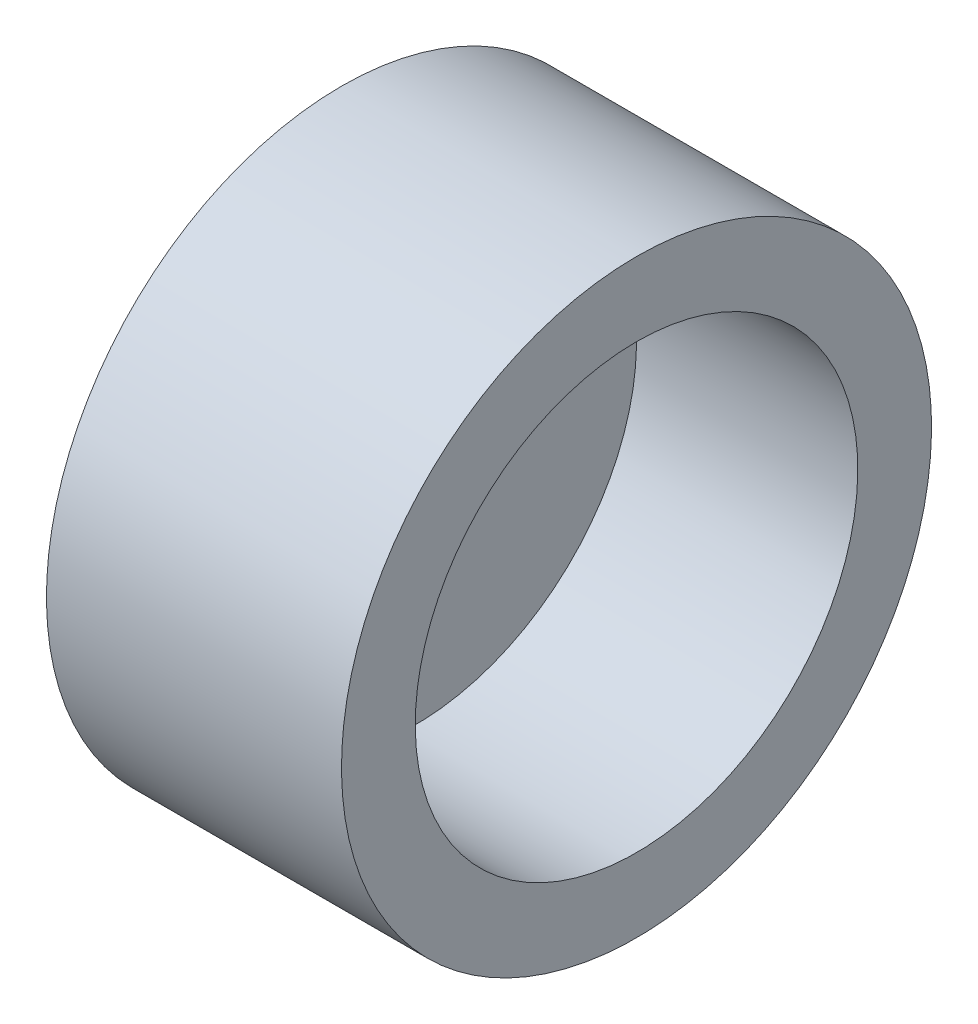
ISO-10303-21;
HEADER;
FILE_DESCRIPTION(('STEP AP214'),'2;1');
FILE_NAME('part.step','',(''),(''),'','','');
FILE_SCHEMA(('AUTOMOTIVE_DESIGN { 1 0 10303 214 1 1 1 1 }'));
ENDSEC;
DATA;
#1=APPLICATION_CONTEXT('core data for automotive mechanical design processes');
#2=APPLICATION_PROTOCOL_DEFINITION('international standard','automotive_design',2000,#1);
#3=PRODUCT_CONTEXT('',#1,'mechanical');
#4=PRODUCT('Part','Part','',(#3));
#5=PRODUCT_RELATED_PRODUCT_CATEGORY('part','',(#4));
#6=PRODUCT_DEFINITION_FORMATION('','',#4);
#7=PRODUCT_DEFINITION_CONTEXT('part definition',#1,'design');
#8=PRODUCT_DEFINITION('design','',#6,#7);
#9=PRODUCT_DEFINITION_SHAPE('','',#8);
#10=(LENGTH_UNIT() NAMED_UNIT(*) SI_UNIT(.MILLI.,.METRE.));
#11=(NAMED_UNIT(*) PLANE_ANGLE_UNIT() SI_UNIT($,.RADIAN.));
#12=(NAMED_UNIT(*) SI_UNIT($,.STERADIAN.) SOLID_ANGLE_UNIT());
#13=UNCERTAINTY_MEASURE_WITH_UNIT(LENGTH_MEASURE(1.E-05),#10,'distance_accuracy_value','');
#14=(GEOMETRIC_REPRESENTATION_CONTEXT(3) GLOBAL_UNCERTAINTY_ASSIGNED_CONTEXT((#13)) GLOBAL_UNIT_ASSIGNED_CONTEXT((#10,
#11,#12)) REPRESENTATION_CONTEXT('',''));
#15=CARTESIAN_POINT('',(0.,0.,0.));
#16=DIRECTION('',(0.,0.,1.));
#17=DIRECTION('',(1.,0.,0.));
#18=AXIS2_PLACEMENT_3D('',#15,#16,#17);
#19=CARTESIAN_POINT('',(-25.4,0.,0.));
#20=DIRECTION('',(-1.,0.,0.));
#21=DIRECTION('',(0.,-1.,0.));
#22=AXIS2_PLACEMENT_3D('',#19,#20,#21);
#23=PLANE('',#22);
#24=CARTESIAN_POINT('',(-25.4,0.,0.));
#25=DIRECTION('',(-1.,0.,0.));
#26=DIRECTION('',(0.,0.,1.));
#27=AXIS2_PLACEMENT_3D('',#24,#25,#26);
#28=CIRCLE('',#27,6.604);
#29=CARTESIAN_POINT('',(-25.4,0.,6.604));
#30=VERTEX_POINT('',#29);
#31=EDGE_CURVE('E56',#30,#30,#28,.T.);
#32=ORIENTED_EDGE('',*,*,#31,.F.);
#33=EDGE_LOOP('',(#32));
#34=FACE_BOUND('',#33,.T.);
#35=CARTESIAN_POINT('',(-25.4,0.,0.));
#36=DIRECTION('',(1.,0.,0.));
#37=DIRECTION('',(0.,1.,0.));
#38=AXIS2_PLACEMENT_3D('',#35,#36,#37);
#39=CIRCLE('',#38,25.4);
#40=CARTESIAN_POINT('',(-25.4,25.4,0.));
#41=VERTEX_POINT('',#40);
#42=EDGE_CURVE('E10',#41,#41,#39,.T.);
#43=ORIENTED_EDGE('',*,*,#42,.F.);
#44=EDGE_LOOP('',(#43));
#45=FACE_BOUND('',#44,.T.);
#46=ADVANCED_FACE('F40',(#34,#45),#23,.T.);
#47=CARTESIAN_POINT('',(-19.05,0.,0.));
#48=DIRECTION('',(1.,0.,0.));
#49=DIRECTION('',(0.,1.,0.));
#50=AXIS2_PLACEMENT_3D('',#47,#48,#49);
#51=CYLINDRICAL_SURFACE('',#50,25.4);
#52=ORIENTED_EDGE('',*,*,#42,.T.);
#53=EDGE_LOOP('',(#52));
#54=FACE_BOUND('',#53,.T.);
#55=CARTESIAN_POINT('',(0.,0.,0.));
#56=DIRECTION('',(1.,0.,0.));
#57=DIRECTION('',(0.,1.,0.));
#58=AXIS2_PLACEMENT_3D('',#55,#56,#57);
#59=CIRCLE('',#58,25.4);
#60=CARTESIAN_POINT('',(0.,25.4,0.));
#61=VERTEX_POINT('',#60);
#62=EDGE_CURVE('E42',#61,#61,#59,.T.);
#63=ORIENTED_EDGE('',*,*,#62,.F.);
#64=EDGE_LOOP('',(#63));
#65=FACE_BOUND('',#64,.T.);
#66=ADVANCED_FACE('F70',(#54,#65),#51,.T.);
#67=CARTESIAN_POINT('',(0.,25.4,0.));
#68=DIRECTION('',(1.,0.,0.));
#69=DIRECTION('',(0.,1.,0.));
#70=AXIS2_PLACEMENT_3D('',#67,#68,#69);
#71=PLANE('',#70);
#72=ORIENTED_EDGE('',*,*,#62,.T.);
#73=EDGE_LOOP('',(#72));
#74=FACE_BOUND('',#73,.T.);
#75=CARTESIAN_POINT('',(0.,0.,0.));
#76=DIRECTION('',(1.,0.,0.));
#77=DIRECTION('',(0.,1.,0.));
#78=AXIS2_PLACEMENT_3D('',#75,#76,#77);
#79=CIRCLE('',#78,19.05);
#80=CARTESIAN_POINT('',(0.,19.05,0.));
#81=VERTEX_POINT('',#80);
#82=EDGE_CURVE('E48',#81,#81,#79,.T.);
#83=ORIENTED_EDGE('',*,*,#82,.F.);
#84=EDGE_LOOP('',(#83));
#85=FACE_BOUND('',#84,.T.);
#86=ADVANCED_FACE('F71',(#74,#85),#71,.T.);
#87=CARTESIAN_POINT('',(-19.05,0.,0.));
#88=DIRECTION('',(1.,0.,0.));
#89=DIRECTION('',(0.,1.,0.));
#90=AXIS2_PLACEMENT_3D('',#87,#88,#89);
#91=CYLINDRICAL_SURFACE('',#90,19.05);
#92=ORIENTED_EDGE('',*,*,#82,.T.);
#93=EDGE_LOOP('',(#92));
#94=FACE_BOUND('',#93,.T.);
#95=CARTESIAN_POINT('',(-19.05,0.,0.));
#96=DIRECTION('',(1.,0.,0.));
#97=DIRECTION('',(0.,1.,0.));
#98=AXIS2_PLACEMENT_3D('',#95,#96,#97);
#99=CIRCLE('',#98,19.05);
#100=CARTESIAN_POINT('',(-19.05,19.05,0.));
#101=VERTEX_POINT('',#100);
#102=EDGE_CURVE('E52',#101,#101,#99,.T.);
#103=ORIENTED_EDGE('',*,*,#102,.F.);
#104=EDGE_LOOP('',(#103));
#105=FACE_BOUND('',#104,.T.);
#106=ADVANCED_FACE('F80',(#94,#105),#91,.F.);
#107=CARTESIAN_POINT('',(-19.05,0.,0.));
#108=DIRECTION('',(1.,0.,0.));
#109=DIRECTION('',(0.,1.,0.));
#110=AXIS2_PLACEMENT_3D('',#107,#108,#109);
#111=PLANE('',#110);
#112=CARTESIAN_POINT('',(-19.05,0.,0.));
#113=DIRECTION('',(1.,0.,0.));
#114=DIRECTION('',(0.,1.,0.));
#115=AXIS2_PLACEMENT_3D('',#112,#113,#114);
#116=CIRCLE('',#115,3.429);
#117=CARTESIAN_POINT('',(-19.05,3.429,0.));
#118=VERTEX_POINT('',#117);
#119=EDGE_CURVE('E37',#118,#118,#116,.T.);
#120=ORIENTED_EDGE('',*,*,#119,.F.);
#121=EDGE_LOOP('',(#120));
#122=FACE_BOUND('',#121,.T.);
#123=ORIENTED_EDGE('',*,*,#102,.T.);
#124=EDGE_LOOP('',(#123));
#125=FACE_BOUND('',#124,.T.);
#126=ADVANCED_FACE('F84',(#122,#125),#111,.T.);
#127=CARTESIAN_POINT('',(-25.4,0.,0.));
#128=DIRECTION('',(-1.,0.,0.));
#129=DIRECTION('',(0.,0.,1.));
#130=AXIS2_PLACEMENT_3D('',#127,#128,#129);
#131=CYLINDRICAL_SURFACE('',#130,3.429);
#132=ORIENTED_EDGE('',*,*,#119,.T.);
#133=EDGE_LOOP('',(#132));
#134=FACE_BOUND('',#133,.T.);
#135=CARTESIAN_POINT('',(-21.7475803070733,0.,0.));
#136=DIRECTION('',(-1.,0.,0.));
#137=DIRECTION('',(0.,0.,1.));
#138=AXIS2_PLACEMENT_3D('',#135,#136,#137);
#139=CIRCLE('',#138,3.429);
#140=CARTESIAN_POINT('',(-21.7475803070733,0.,3.429));
#141=VERTEX_POINT('',#140);
#142=EDGE_CURVE('E57',#141,#141,#139,.T.);
#143=ORIENTED_EDGE('',*,*,#142,.T.);
#144=EDGE_LOOP('',(#143));
#145=FACE_BOUND('',#144,.T.);
#146=ADVANCED_FACE('F88',(#134,#145),#131,.F.);
#147=CARTESIAN_POINT('',(-25.4,0.,0.));
#148=DIRECTION('',(-1.,0.,0.));
#149=DIRECTION('',(0.,0.,1.));
#150=AXIS2_PLACEMENT_3D('',#147,#148,#149);
#151=CONICAL_SURFACE('',#150,6.604,0.715584993317675);
#152=ORIENTED_EDGE('',*,*,#142,.F.);
#153=EDGE_LOOP('',(#152));
#154=FACE_BOUND('',#153,.T.);
#155=ORIENTED_EDGE('',*,*,#31,.T.);
#156=EDGE_LOOP('',(#155));
#157=FACE_BOUND('',#156,.T.);
#158=ADVANCED_FACE('F62',(#154,#157),#151,.F.);
#159=CLOSED_SHELL('',(#46,#66,#86,#106,#126,#146,#158));
#160=MANIFOLD_SOLID_BREP('B2',#159);
#161=ADVANCED_BREP_SHAPE_REPRESENTATION('',(#18,#160),#14);
#162=SHAPE_DEFINITION_REPRESENTATION(#9,#161);
ENDSEC;
END-ISO-10303-21;
